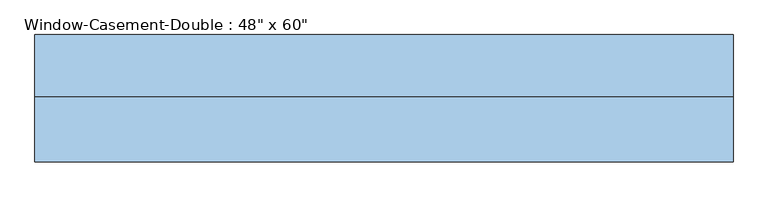
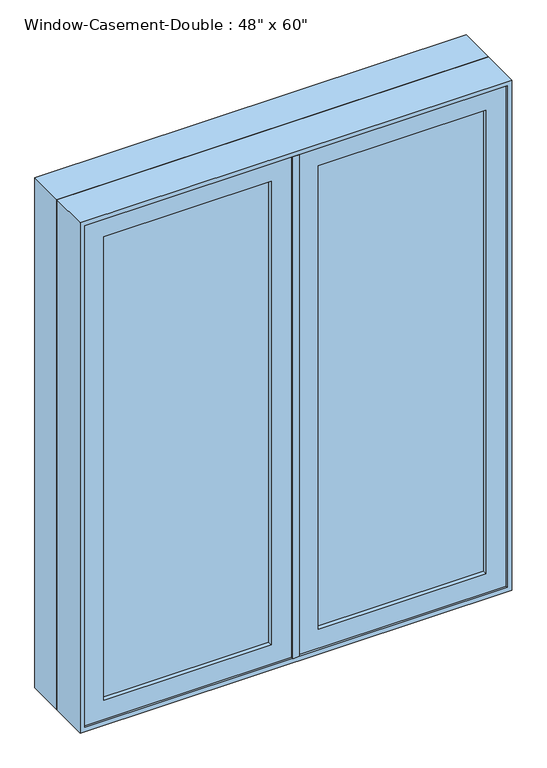
"""IFC4 building model written with IfcOpenShell, lengths in millimetres: window geometry."""

from ifc_helpers import new_model, si_unit, frame, origin, place, context, project, spatial, polyline, outline, extrude, faceted_brep, source, transform, mapped, element, save


def window_f2c349b1(model_context):
    return source(origin(), model_context, "Body", "SolidModel", [
        faceted_brep([(9.525, -120.65, 2425.7), (9.525, -69.85, 2425.7), (-9.525, -69.85, 2425.7), (-9.525, -120.65, 2425.7), (9.525, -120.65, 927.1), (-9.525, -120.65, 927.1), (-9.525, -69.85, 927.1), (9.525, -69.85, 927.1), (-9.525, -69.85, 2406.65), (-9.525, -69.85, 946.15), (-30.1625, -69.85, 2406.65), (-30.1625, -69.85, 946.15), (-30.1625, -6.35, 2406.65), (-30.1625, -6.35, 946.15), (30.1625, -6.35, 2406.65), (30.1625, -6.35, 946.15), (30.1625, -69.85, 2406.65), (30.1625, -69.85, 946.15), (9.525, -69.85, 2406.65), (9.525, -69.85, 946.15)], [[[0, 1, 2, 3]], [[4, 5, 6, 7]], [[3, 5, 4, 0]], [[2, 8, 9, 6, 5, 3]], [[8, 10, 11, 9]], [[10, 12, 13, 11]], [[12, 14, 15, 13]], [[14, 16, 17, 15]], [[16, 18, 19, 17]], [[0, 4, 7, 19, 18, 1]], [[8, 2, 1, 18]], [[19, 7, 6, 9]], [[9, 11, 13, 15, 17, 19]], [[18, 16, 14, 12, 10, 8]]]),
        extrude(outline(polyline([(-66.675, -101.6), (-539.75, -101.6), (-539.75, -95.25), (-66.675, -95.25), (-66.675, -101.6)])), frame((0.0, 0.0, 984.25), z_axis=(0.0, 0.0, 1.0), x_axis=(1.0, 0.0, 0.0)), (0.0, 0.0, 1.0), 1384.3),
        extrude(outline(polyline([(-539.75, -82.55), (-66.675, -82.55), (-66.675, -88.9), (-539.75, -88.9), (-539.75, -82.55)])), frame((0.0, 0.0, 984.25), z_axis=(0.0, 0.0, 1.0), x_axis=(1.0, 0.0, 0.0)), (0.0, 0.0, 1.0), 1384.3),
        extrude(outline(polyline([(539.75, -101.6), (66.675, -101.6), (66.675, -95.25), (539.75, -95.25), (539.75, -101.6)])), frame((0.0, 0.0, 984.25), z_axis=(0.0, 0.0, 1.0), x_axis=(1.0, 0.0, 0.0)), (0.0, 0.0, 1.0), 1384.3),
        extrude(outline(polyline([(66.675, -82.55), (539.75, -82.55), (539.75, -88.9), (66.675, -88.9), (66.675, -82.55)])), frame((0.0, 0.0, 984.25), z_axis=(0.0, 0.0, 1.0), x_axis=(1.0, 0.0, 0.0)), (0.0, 0.0, 1.0), 1384.3),
        extrude(outline(polyline([(2425.7, -9.525), (2425.7, -596.9), (927.1, -596.9), (927.1, -9.525), (2425.7, -9.525)]), holes=[polyline([(2368.55, -539.75), (2368.55, -66.675), (984.25, -66.675), (984.25, -539.75), (2368.55, -539.75)])]), frame((0.0, -114.3, 0.0), z_axis=(0.0, 1.0, 0.0), x_axis=(0.0, 0.0, 1.0)), (0.0, 0.0, 1.0), 44.45),
        extrude(outline(polyline([(927.1, 9.525), (927.1, 596.9), (2425.7, 596.9), (2425.7, 9.525), (927.1, 9.525)]), holes=[polyline([(984.25, 539.75), (984.25, 66.675), (2368.55, 66.675), (2368.55, 539.75), (984.25, 539.75)])]), frame((0.0, -114.3, 0.0), z_axis=(0.0, 1.0, 0.0), x_axis=(0.0, 0.0, 1.0)), (0.0, 0.0, 1.0), 44.45),
        extrude(outline(polyline([(2438.4, -609.6), (914.4, -609.6), (914.4, 609.6), (2438.4, 609.6), (2438.4, -609.6)]), holes=[polyline([(2419.35, 590.55), (933.45, 590.55), (933.45, -590.55), (2419.35, -590.55), (2419.35, 590.55)])]), frame((0.0, -6.35, 0.0), z_axis=(0.0, 1.0, 0.0), x_axis=(0.0, 0.0, 1.0)), (0.0, 0.0, 1.0), 107.95),
        faceted_brep([(577.85, -69.85, 2406.65), (-577.85, -69.85, 2406.65), (-577.85, -6.35, 2406.65), (577.85, -6.35, 2406.65), (596.9, -120.65, 2425.7), (-596.9, -120.65, 2425.7), (-596.9, -69.85, 2425.7), (596.9, -69.85, 2425.7), (609.6, -6.35, 2438.4), (-609.6, -6.35, 2438.4), (-609.6, -120.65, 2438.4), (609.6, -120.65, 2438.4), (-577.85, -69.85, 946.15), (-577.85, -6.35, 946.15), (-596.9, -120.65, 927.1), (-596.9, -69.85, 927.1), (-609.6, -6.35, 914.4), (-609.6, -120.65, 914.4), (577.85, -69.85, 946.15), (577.85, -6.35, 946.15), (596.9, -120.65, 927.1), (596.9, -69.85, 927.1), (609.6, -6.35, 914.4), (609.6, -120.65, 914.4)], [[[0, 1, 2, 3]], [[4, 5, 6, 7]], [[8, 9, 10, 11]], [[1, 12, 13, 2]], [[5, 14, 15, 6]], [[9, 16, 17, 10]], [[12, 18, 19, 13]], [[14, 20, 21, 15]], [[16, 22, 23, 17]], [[9, 8, 22, 16], [3, 2, 13, 19]], [[18, 0, 3, 19]], [[7, 6, 15, 21], [1, 0, 18, 12]], [[20, 4, 7, 21]], [[22, 8, 11, 23]], [[11, 10, 17, 23], [5, 4, 20, 14]]]),
    ])


if __name__ == "__main__":
    model = new_model("IFC4")
    model_context = context("Model", 3, world=origin())
    ifc_project = project(units=[si_unit("LENGTHUNIT", "METRE", prefix="MILLI")], contexts=[model_context])
    site = spatial("IfcSite", under=ifc_project)
    building = spatial("IfcBuilding", under=site)
    placement = place(None, origin())
    window_shape = window_f2c349b1(model_context)
    element("IfcWindow", 1, ObjectType="Window-Casement-Double : 48\" x 60\"", at=placement, inside=building, context=model_context, shape_type="MappedRepresentation", body=[
        mapped(window_shape, transform((0.0, 0.0, 0.0), x_axis=(1.0, 0.0, 0.0), y_axis=(0.0, 1.0, 0.0), z_axis=(0.0, 0.0, 1.0))),
    ])
    save(model, "model.ifc")

# Revit data of these elements
# Type "Window-Casement-Double : 48\" x 60\""
#   Type Mark = "16"
#   Fire Rating = "0.5h"
#   Assembly Code = "B2020100"
#   Analytic Construction = "Double glazing - domestic"
#   Frame Extension [instance default] = 0' - 0 1/4"
#   Window Inset [instance default] = 0' - 0"
#   Wall Thickness [instance default] = 0' - 6"
#   Interior Wall Closure [instance default] = 0' - 2 1/4"
#   Half Width = 2' - 0"
#   Visual Light Transmittance = 0.81
#   Thermal Resistance (R) = 1.8146 (h·ft²·°F)/BTU
#   Solar Heat Gain Coefficient = 0.76
#   Rough Width = 4' - 0 1/2"
#   Rough Height = 5' - 0 1/2"
#   Height = 5' - 0"
#   Heat Transfer Coefficient (U) = 0.5511 BTU/(h·ft²·°F)
#   Exterior Wall Closure [instance default] = 0' - 1 1/4"
#   Extension Jamb [instance default] = 0' - 2 1/4"
#   Default Sill Height = 3' - 0"
#   Width = 4' - 0"
#   Define Thermal Properties by = 0
#   Muntin Visibility = yes
#   Interior Trim Visibility [instance default] = yes
#   Exterior Trim Visibility [instance default] = yes
#   Extension Jamb Visibility [instance default] = yes
#   Interior Trim Material = Wood - Stained
#   Muntin Pattern = Muntin Pattern_2x2 : Muntin Pattern_2x2
#   Interior Trim = Trim-Window-Interior-Flat : Picture Frame
#   Interior Frame Material = Wood - Stained
#   Glass Panel Material = Glass
#   Exterior Trim Material = Clad - White
#   Exterior Trim = Trim-Window-Exterior-Flat : with Sill
#   Exterior Frame Material = Clad - White
#   Wall Closure = (empty or 0)
# Element 1 (IfcWindow, "Window-Casement-Double : 48\" x 60\"")
#   Wall Thickness = 0' - 8"
#   Extension Jamb = 0' - 4 1/4"
#   Materials on its faces: "Wood - Stained", "Glass", "Clad - White"
# Materials
#   "Wood - Stained": class "Wood", colour RGB 224 178 126, transparency 0, Cost = 0
#   "Glass": class "Glass", colour RGB 0 128 192, transparency 0.75, Description = "Soda Lime Glass", Cost = 0
#   "Clad - White": class "Wood", colour RGB 242 242 238, transparency 0, Cost = 0
